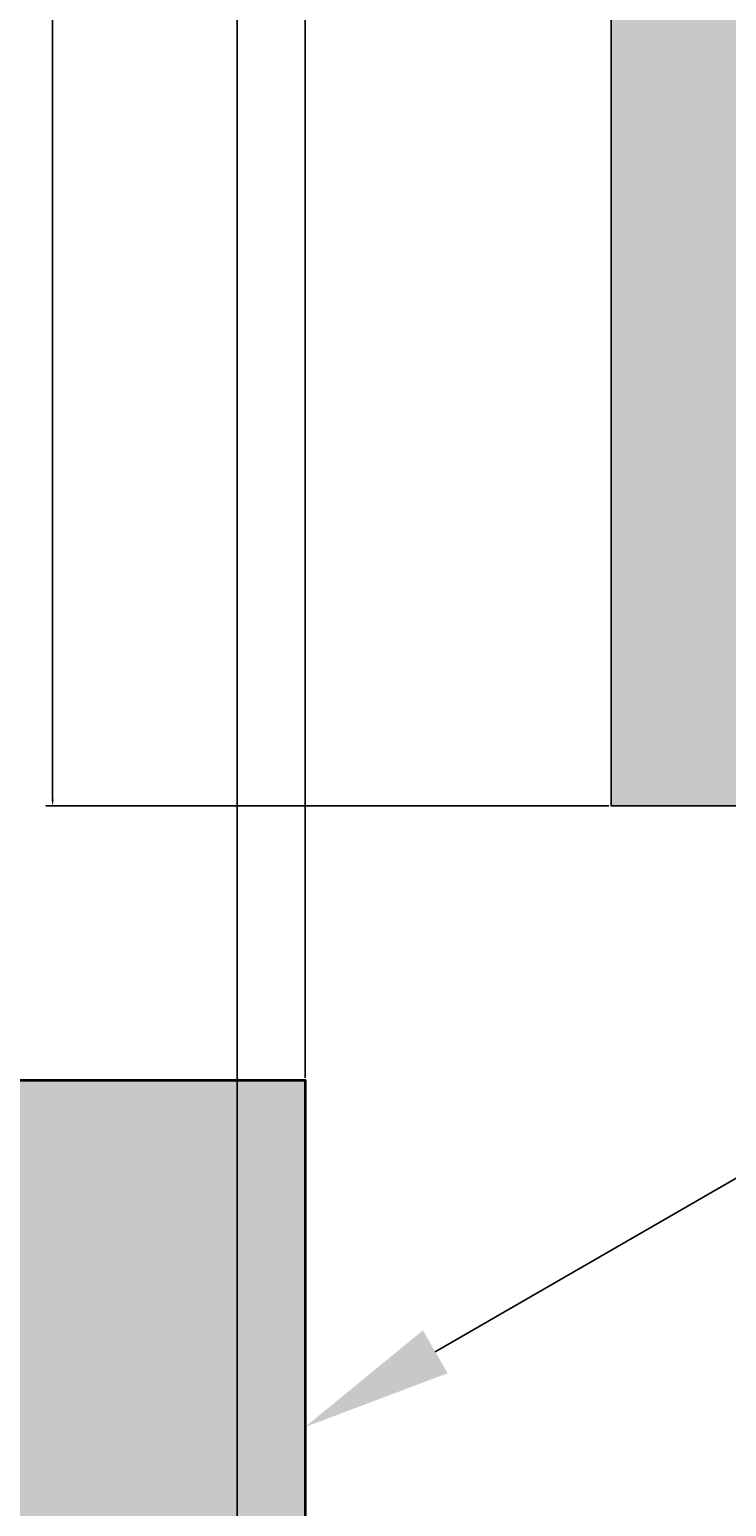
# Model space of a CAD drawing. Units: millimetres. Extents: x -11 to 280, y -4 to 208.
# Tile 8 of 55: x 24 to 42, y 87 to 126. Entities that reach past the tile are written whole.
import ezdxf
from ezdxf import colors
from ezdxf.entities.mleader import LeaderData, LeaderLine
from ezdxf.math import Vec2, Vec3

# ---------------------------------------------------------------- set-up
doc = ezdxf.new("R2010")
doc.units = ezdxf.units.MM
for name, color, linetype, lineweight in [('M-ANNO-TEXT', 7, 'Continuous', 18), ('M-DIMS', 2, 'Continuous', 18), ('M-HYDR-EQPM', 7, 'Continuous', 35), ('M-HYDR-EQPM-PATT', 252, 'Continuous', 13), ('M-HYDR-SUCT', 7, 'Continuous', 25)]:
    doc.layers.add(name, color=color, linetype=linetype, lineweight=lineweight)
doc.layers.add('M-HYDR-SUCT-PATT', color=221, linetype='Continuous', lineweight=13, true_color=0xff7fdf)
doc.styles.get("Standard").update_dxf_attribs({"font": 'arial.ttf'})
doc.dimstyles.get("Standard").update_dxf_attribs({"dimtxt": 0.18, "dimasz": 0.18, "dimexe": 0.18, "dimexo": 0.0625, "dimgap": 0.09, "dimtad": 0, "dimtih": 1, "dimtoh": 1, "dimdec": 4, "dimzin": 0, "dimdsep": 46, "dimtxsty": 'Standard', "dimcen": 0.09, "dimadec": 0, "dimazin": 0, "dimtfac": 1, "dimtdec": 4, "dimtofl": 0, "dimtmove": 0, "dimatfit": 3, "dimfxl": 1, "dimtolj": 1, "dimtzin": 0, "dimarcsym": 0})

# ---------------------------------------------------------------- blocks, each defined once
blk = doc.blocks.new('*D5')
at = {"layer": 'Defpoints', "color": 0, "transparency": 16777216}
for p in [(24.759, 192.645), (-10.087, 11.435), (261.686, 11.435)]:
    blk.add_point(p, dxfattribs=at)
at = {"layer": 'M-DIMS', "color": 0, "lineweight": -2, "transparency": 16777216}
for p, q in [((24.696, 192.645), (-10.267, 192.645)), ((-10.087, 192.465), (-10.087, 102.222)), ((-10.087, 11.615), (-10.087, 101.858)), ((261.624, 11.435), (-10.267, 11.435))]:
    blk.add_line(p, q, dxfattribs=at)
at = {"layer": 'M-DIMS', "color": 0, "transparency": 16777216}
for points in [[(-10.117, 192.465), (-10.057, 192.465), (-10.087, 192.645)], [(-10.117, 11.615), (-10.057, 11.615), (-10.087, 11.435)]]:
    blk.add_solid(points, dxfattribs=at)
at = {"layer": 'M-DIMS', "color": 0, "transparency": 16777216, "insert": (-10.087, 102.04), "char_height": 0.18, "attachment_point": 5}
blk.add_mtext('\\A1;181.2', dxfattribs=at)
blk = doc.blocks.new('*D9')
at = {"layer": 'Defpoints', "color": 0, "transparency": 16777216}
for p in [(78.827, 207.495), (31.006, 98.021), (78.827, 98.149)]:
    blk.add_point(p, dxfattribs=at)
at = {"layer": 'M-DIMS', "color": 0, "lineweight": -2, "transparency": 16777216}
for p, q in [((31.006, 98.084), (31.006, 207.675)), ((31.186, 207.495), (54.52, 207.495)), ((78.647, 207.495), (55.313, 207.495)), ((78.827, 98.212), (78.827, 207.675))]:
    blk.add_line(p, q, dxfattribs=at)
at = {"layer": 'M-DIMS', "color": 0, "transparency": 16777216}
for points in [[(31.186, 207.525), (31.186, 207.465), (31.006, 207.495)], [(78.647, 207.525), (78.647, 207.465), (78.827, 207.495)]]:
    blk.add_solid(points, dxfattribs=at)
at = {"layer": 'M-DIMS', "color": 0, "transparency": 16777216, "insert": (54.917, 207.495), "char_height": 0.18, "attachment_point": 5}
blk.add_mtext('\\A1;47.82', dxfattribs=at)
blk = doc.blocks.new('*D10')
at = {"layer": 'Defpoints', "color": 0, "transparency": 16777216}
for p in [(24.295, 153.977), (39.145, 153.977), (39.145, 105.314)]:
    blk.add_point(p, dxfattribs=at)
at = {"layer": 'M-DIMS', "color": 0, "lineweight": -2, "transparency": 16777216}
for p, q in [((39.083, 153.977), (24.115, 153.977)), ((24.295, 153.797), (24.295, 129.827)), ((24.295, 105.494), (24.295, 129.464)), ((39.083, 105.314), (24.115, 105.314))]:
    blk.add_line(p, q, dxfattribs=at)
at = {"layer": 'M-DIMS', "color": 0, "transparency": 16777216}
for points in [[(24.265, 153.797), (24.325, 153.797), (24.295, 153.977)], [(24.265, 105.494), (24.325, 105.494), (24.295, 105.314)]]:
    blk.add_solid(points, dxfattribs=at)
at = {"layer": 'M-DIMS', "color": 0, "transparency": 16777216, "insert": (24.295, 129.645), "char_height": 0.18, "attachment_point": 5}
blk.add_mtext('\\A1;48.66', dxfattribs=at)
blk = doc.blocks.new('*D23')
at = {"layer": 'Defpoints', "color": 0, "transparency": 16777216}
for p in [(29.201, 153.977), (66.388, 153.977), (66.388, -3.415)]:
    blk.add_point(p, dxfattribs=at)
at = {"layer": 'M-DIMS', "color": 0, "lineweight": -2, "transparency": 16777216}
for p, q in [((29.201, 153.914), (29.201, -3.595)), ((66.388, 153.914), (66.388, -3.595)), ((29.381, -3.415), (47.331, -3.415)), ((66.208, -3.415), (48.258, -3.415))]:
    blk.add_line(p, q, dxfattribs=at)
at = {"layer": 'M-DIMS', "color": 0, "transparency": 16777216}
for points in [[(29.381, -3.385), (29.381, -3.445), (29.201, -3.415)], [(66.208, -3.385), (66.208, -3.445), (66.388, -3.415)]]:
    blk.add_solid(points, dxfattribs=at)
at = {"layer": 'M-DIMS', "color": 0, "transparency": 16777216, "insert": (47.795, -3.415), "char_height": 0.18, "attachment_point": 5}
blk.add_mtext('\\A1;37.186', dxfattribs=at)

msp = doc.modelspace()

# ---------------------------------------------------------------- hatches: boundary and pattern name
at = {"layer": 'M-HYDR-EQPM-PATT'}
h = msp.add_hatch(color=256, dxfattribs=at)
h.set_gradient(color1=(69, 84, 165), color2=(0, 0, 255), tint=1)
h.paths.add_polyline_path([(31.0059, 84.4261), (31.0059, 98.0213), (4.7635, 98.0213), (4.7635, 84.4261)])
at = {"layer": 'M-HYDR-SUCT-PATT'}
h = msp.add_hatch(color=256, dxfattribs=at)
h.set_gradient(color1=(255, 127, 223), color2=(255, 127, 223), tint=1, name='INVCYLINDER')
h.paths.add_polyline_path([(91.3629, 155.4768), (91.3629, 132.4768), (58.3629, 132.4768), (58.3629, 153.9768), (54.8629, 153.9768), (54.8629, 128.9768), (94.8629, 128.9768), (94.8629, 151.9768), (205.5315, 151.9768), (205.5315, 155.4768)])
h.paths.add_polyline_path([(91.3, 114.9452, 1), (78.8273, 114.9452), (78.8273, 108.8141), (42.6453, 108.8141), (42.6453, 153.9768), (39.1453, 153.9768), (39.1453, 105.3141), (78.8273, 105.3141), (78.8273, 98.1491, 1), (91.3, 98.1491), (91.3, 105.3141), (95.5776, 105.3141), (95.5776, 108.8141), (91.3, 108.8141)])
h.paths.add_polyline_path([(228.7, 138.4081), (232.2, 138.4081), (232.2, 144.6609), (228.7, 144.6609)])
h.paths.add_polyline_path([(253.1005, 151.9768, 1), (253.1005, 155.4768), (252.6001, 155.4768), (253.5249, 153.991, -0.1401047), (253.6005, 153.7268, -0.7542249), (252.676, 153.4626), (251.4221, 155.4768), (236.9353, 155.4768), (236.9353, 151.9768)])
h.paths.add_polyline_path([(30.8182, 40.7626), (30.8182, 36.7626), (60.8182, 36.7626), (60.8182, 40.7626)])

# ---------------------------------------------------------------- linework, layer by layer
at = {"layer": 'M-HYDR-EQPM'}
msp.add_lwpolyline([(4.7635, 98.0213), (31.0059, 98.0213), (31.0059, 84.4261), (4.7635, 84.4261)], close=True, dxfattribs=at)
at = {"layer": 'M-HYDR-SUCT'}
msp.add_lwpolyline([(78.8273, 105.3141), (39.1453, 105.3141), (39.1453, 153.9768)], dxfattribs=at)

# ---------------------------------------------------------------- dimensions: what is measured, and where the dimension line sits
at = {"layer": 'M-DIMS'}
for base, p1, p2, override, picture, middle in [((78.8273, 207.495), (31.0059, 98.0213), (78.8273, 98.1491), {"dimdec": 2, "dimlfac": 1, "dimrnd": 0, "dimzin": 0, "dimdsep": 46, "dimlunit": 2}, '*D9', (54.9166, 207.495)), ((66.3875, -3.4154), (29.2015, 153.9768), (66.3875, 153.9768), {"dimdec": 3, "dimlfac": 1, "dimrnd": 0, "dimzin": 0, "dimdsep": 46, "dimlunit": 2}, '*D23', (47.7945, -3.4154))]:
    dim = msp.add_linear_dim(base=base, p1=p1, p2=p2, dimstyle='Standard', override=override, dxfattribs=at)
    dim.commit()
    dim.dimension.update_dxf_attribs({"geometry": picture, "text_midpoint": middle})
for base, p1, p2, override, picture, middle in [((-10.0865, 11.4346), (24.7588, 192.645), (261.6863, 11.4346), {"dimdec": 1, "dimlfac": 1, "dimrnd": 0, "dimzin": 0, "dimdsep": 46, "dimlunit": 2}, '*D5', (-10.0865, 102.0398)), ((24.2953, 153.9768), (39.1453, 105.3141), (39.1453, 153.9768), {"dimdec": 2, "dimlfac": 1, "dimrnd": 0, "dimzin": 0, "dimdsep": 46, "dimlunit": 2}, '*D10', (24.2953, 129.6454))]:
    dim = msp.add_linear_dim(base=base, p1=p1, p2=p2, angle=90, dimstyle='Standard', override=override, dxfattribs=at)
    dim.commit()
    dim.dimension.update_dxf_attribs({"geometry": picture, "text_midpoint": middle})

# ---------------------------------------------------------------- leaders
at = {"layer": 'M-ANNO-TEXT'}
ml = msp.add_multileader_mtext('Standard', dxfattribs=at)
ml.set_content('FILTER', color=256)
ml.set_leader_properties()
ml.build(insert=Vec2(0, 0))
ctx = ml.context
ctx.base_point, ctx.plane_origin = Vec3(50.7635, 95.5863), Vec3(31.0059, 88.798)
notes = []
notes.append((ctx, [(0, (1, 1, 0), (42.7635, 95.5863), (1, 0), 8, [(0, [(31.0059, 88.798)], 0, [])])]))
ctx.mtext.insert, ctx.mtext.flow_direction = Vec3(52.7635, 97.5863), 5
for ctx, leaders in notes:
    for number, flags, end, landing, length, lines in leaders:
        leader = LeaderData()
        leader.index, (leader.has_last_leader_line, leader.has_dogleg_vector, leader.attachment_direction) = number, flags
        leader.last_leader_point, leader.dogleg_vector, leader.dogleg_length = Vec3(end), Vec3(landing), length
        for number, points, colour, breaks in lines:
            line = LeaderLine()
            line.index, line.vertices, line.color, line.breaks = number, Vec3.list(points), colors.encode_raw_color(colour), breaks
            leader.lines.append(line)
        ctx.leaders.append(leader)

doc.saveas('drawing.dxf')
